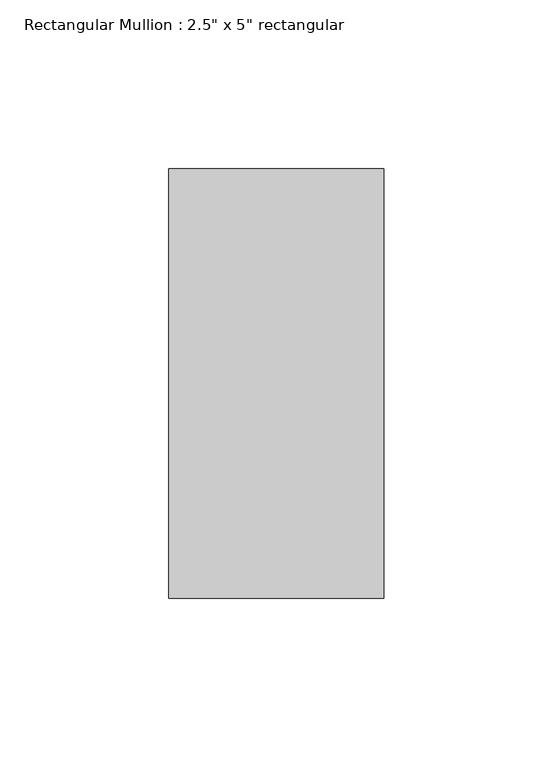
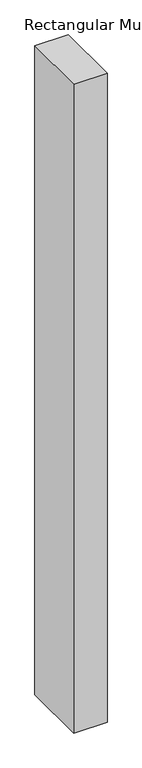
"""IFC4 building model written with IfcOpenShell, lengths in millimetres: member geometry."""

from ifc_helpers import new_model, si_unit, frame, origin, place, context, project, spatial, polyline, outline, extrude, source, transform, mapped, element, save


def member_9869c819(model_context):
    return source(origin(), model_context, "Body", "SweptSolid", [
        extrude(outline(polyline([(31.75, 63.5), (31.75, -63.5), (-31.75, -63.5), (-31.75, 63.5), (31.75, 63.5)])), frame((0.0, 0.0, -1301.6187331), z_axis=(0.0, 0.0, 1.0), x_axis=(1.0, 0.0, 0.0)), (0.0, 0.0, 1.0), 1301.6187331),
    ])


if __name__ == "__main__":
    model = new_model("IFC4")
    model_context = context("Model", 3, world=origin())
    ifc_project = project(units=[si_unit("LENGTHUNIT", "METRE", prefix="MILLI")], contexts=[model_context])
    site = spatial("IfcSite", under=ifc_project)
    building = spatial("IfcBuilding", under=site)
    placement = place(None, origin())
    member_shape = member_9869c819(model_context)
    element("IfcMember", 1, ObjectType="Rectangular Mullion : 2.5\" x 5\" rectangular", at=placement, inside=building, context=model_context, shape_type="MappedRepresentation", body=[
        mapped(member_shape, transform((0.0, 0.0, 0.0), x_axis=(1.0, 0.0, 0.0), y_axis=(0.0, 1.0, 0.0), z_axis=(0.0, 0.0, 1.0))),
    ])
    save(model, "model.ifc")

# Revit data of these elements
# Type "Rectangular Mullion : 2.5\" x 5\" rectangular"
#   built-in parameter 1007304 = 0.416667 (stored number, unit not read)
#   built-in parameter 1007301 = 0.104167 (stored number, unit not read)
#   built-in parameter 1007300 = 0.104167 (stored number, unit not read)
# Element 1 (IfcMember, "Rectangular Mullion : 2.5\" x 5\" rectangular")
#   Materials on its faces: "Aluminum"
# Materials
#   "Aluminum": class "Metal", colour RGB 247 247 247, transparency 0, Description = "Aluminum 6061", Cost = 0
